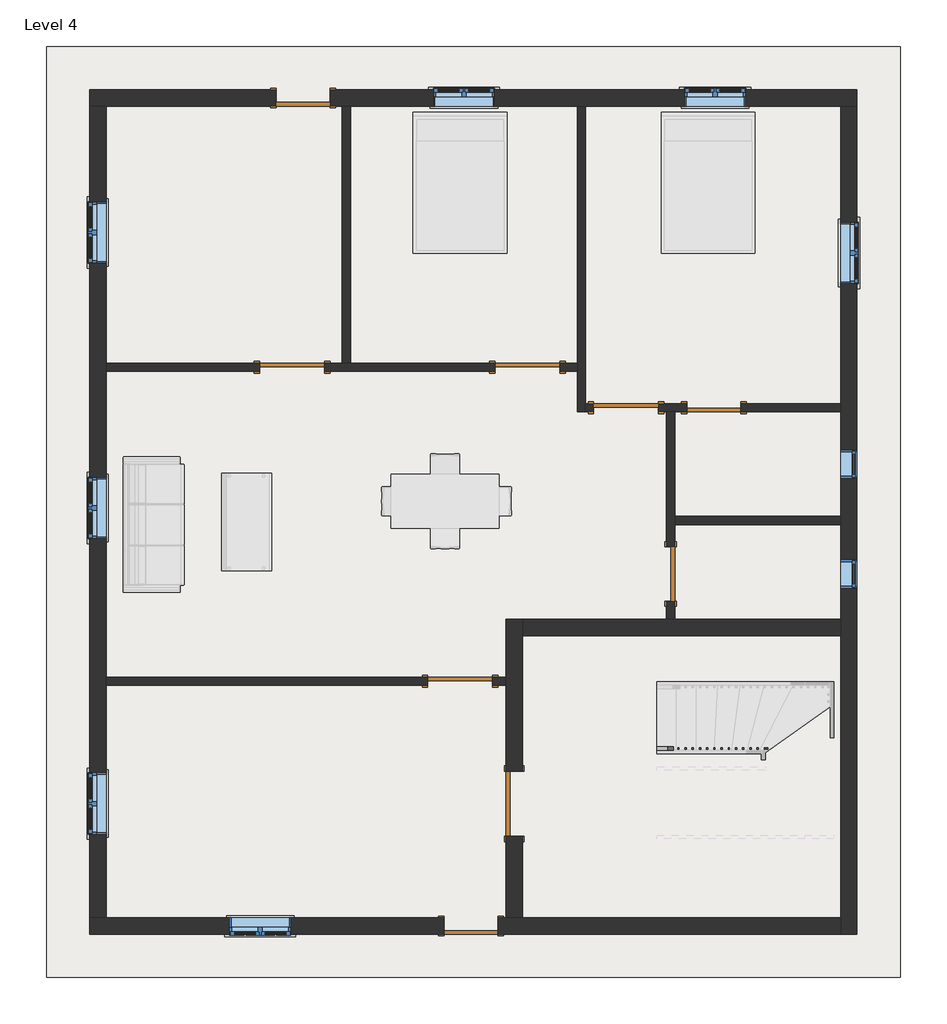
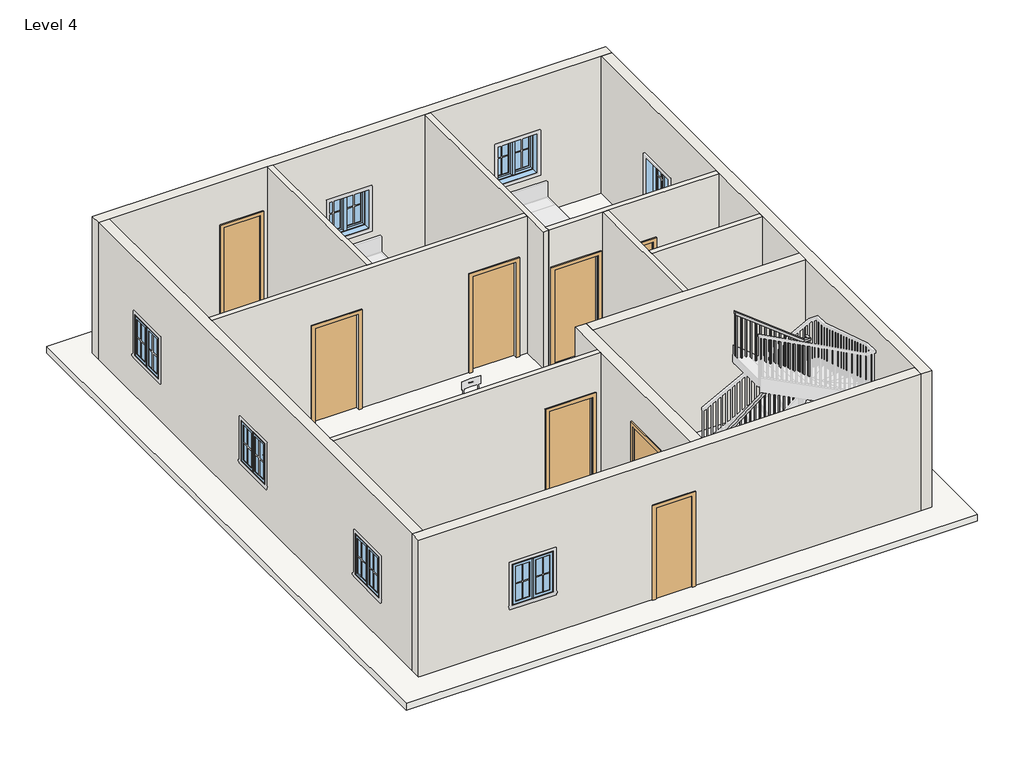
# One storey, part 1 of 2: 13 walls, 9 doors, 9 windows, 1 railing, 1 roof.
"""IFC4 building model written with IfcOpenShell, lengths in millimetres."""

from ifc_helpers import new_model, si_unit, frame, origin, place, context, project, spatial, polyline, outline, extrude, faceted_brep, transform, mapped, element, save
from components import door_85036156, door_d8f5dbb5, door_a1484949, door_e5f9f3c4, door_305aa2a5, door_0ca8825f, window_aa618e30, window_339605e1

model = new_model("IFC4")

# Units and contexts
model_context = context("Model", 3, world=origin())
ifc_project = project(units=[si_unit("LENGTHUNIT", "METRE", prefix="MILLI")], contexts=[model_context])

# Site, building, storey
site = spatial("IfcSite", under=ifc_project)
building = spatial("IfcBuilding", under=site)
storey = spatial("IfcBuildingStorey", under=building, Name="Level 4", Elevation=6400.8)

# Doors
placement = place(None, origin())
door_shape = door_85036156(model_context)
element("IfcDoor", 1, ObjectType="Single-Flush : 30\" x 80\"", at=placement, inside=storey, context=model_context, shape_type="MappedRepresentation", body=[
    mapped(door_shape, transform((-3639.3817864, 7024.9034997, 6400.8), x_axis=(1.0, 0.0, 0.0), y_axis=(0.0, 1.0, 0.0), z_axis=(0.0, 0.0, 1.0))),
])
door_2_shape = door_d8f5dbb5(model_context)
element("IfcDoor", 2, ObjectType="Single-Flush : 30\" x 80\"", at=placement, inside=storey, context=model_context, shape_type="MappedRepresentation", body=[
    mapped(door_2_shape, transform((2149.2782136, 2662.4534997, 6400.8), x_axis=(-1.0, 0.0, 0.0), y_axis=(0.0, -1.0, 0.0), z_axis=(0.0, 0.0, 1.0))),
])
element("IfcDoor", 3, ObjectType="Single-Flush : 30\" x 80\"", at=placement, inside=storey, context=model_context, shape_type="MappedRepresentation", body=[
    mapped(door_2_shape, transform((1539.6782136, 322.4784997, 6400.8), x_axis=(0.0, -1.0, 0.0), y_axis=(1.0, 0.0, 0.0), z_axis=(0.0, 0.0, 1.0))),
])
door_3_shape = door_a1484949(model_context)
element("IfcDoor", 4, ObjectType="Single-Flush : 30\" x 80\"", at=placement, inside=storey, context=model_context, shape_type="MappedRepresentation", body=[
    mapped(door_3_shape, transform((-1273.3717864, -4633.6965003, 6400.8), x_axis=(-1.0, 0.0, 0.0), y_axis=(0.0, -1.0, 0.0), z_axis=(0.0, 0.0, 1.0))),
])
door_4_shape = door_e5f9f3c4(model_context)
element("IfcDoor", 5, ObjectType="Single-Flush : 36\" x 84\"", at=placement, inside=storey, context=model_context, shape_type="MappedRepresentation", body=[
    mapped(door_4_shape, transform((-477.0817864, 3233.9534997, 6400.8), x_axis=(1.0, 0.0, 0.0), y_axis=(0.0, 1.0, 0.0), z_axis=(0.0, 0.0, 1.0))),
])
element("IfcDoor", 6, ObjectType="Single-Flush : 36\" x 84\"", at=placement, inside=storey, context=model_context, shape_type="MappedRepresentation", body=[
    mapped(door_4_shape, transform((-3791.7817864, 3233.9534997, 6400.8), x_axis=(1.0, 0.0, 0.0), y_axis=(0.0, 1.0, 0.0), z_axis=(0.0, 0.0, 1.0))),
])
element("IfcDoor", 7, ObjectType="Single-Flush : 36\" x 84\"", at=placement, inside=storey, context=model_context, shape_type="MappedRepresentation", body=[
    mapped(door_4_shape, transform((-1425.7717864, -1188.1865003, 6400.8), x_axis=(1.0, 0.0, 0.0), y_axis=(0.0, 1.0, 0.0), z_axis=(0.0, 0.0, 1.0))),
])
door_5_shape = door_305aa2a5(model_context)
element("IfcDoor", 8, ObjectType="Single-Flush : 36\" x 84\"", at=placement, inside=storey, context=model_context, shape_type="MappedRepresentation", body=[
    mapped(door_5_shape, transform((912.2982136, 2662.4534997, 6400.8), x_axis=(-1.0, 0.0, 0.0), y_axis=(0.0, -1.0, 0.0), z_axis=(0.0, 0.0, 1.0))),
])
door_6_shape = door_0ca8825f(model_context)
element("IfcDoor", 9, ObjectType="Single-Flush : 36\" x 84\"", at=placement, inside=storey, context=model_context, shape_type="MappedRepresentation", body=[
    mapped(door_6_shape, transform((-663.7717864, -2910.9415003, 6400.8), x_axis=(0.0, 1.0, 0.0), y_axis=(-1.0, 0.0, 0.0), z_axis=(0.0, 0.0, 1.0))),
])

# Railing
element("IfcRailing", 10, ObjectType="Handrail - Rectangular", at=placement, inside=storey, context=model_context, shape_type="SolidModel", body=[
    faceted_brep([(1342.8282136, -2108.9365003, 7484.5333333), (1342.8282136, -2108.9365003, 7420.2000346), (1342.8282136, -2159.7365003, 7420.2000346), (1342.8282136, -2159.7365003, 7484.5333333), (2794.3599055, -2108.9365003, 8612.4191036), (2845.1599055, -2108.9365003, 8587.5590024), (2845.1599055, -2159.7365003, 8587.5590024), (2794.3599055, -2159.7365003, 8612.4191036), (2794.3599055, -2108.9365003, 8815.4281882), (2845.1599055, -2108.9365003, 8764.6281882), (2845.1599055, -2159.7365003, 8764.6281882), (2794.3599055, -2159.7365003, 8815.4281882), (2921.3599055, -2108.9365003, 8815.4281882), (2921.3599055, -2108.9365003, 8764.6281882), (2870.5599055, -2159.7365003, 8764.6281882), (2870.5599055, -2159.7365003, 8815.4281882), (2921.3599055, -2235.9365003, 8815.4281882), (2921.3599055, -2265.0578342, 8764.6281882), (2870.5599055, -2265.0578342, 8764.6281882), (2870.5599055, -2235.9365003, 8815.4281882), (2921.3599055, -2362.9365003, 9032.3051451), (2921.3599055, -2413.7365003, 9018.5256424), (2870.5599055, -2413.7365003, 9018.5256424), (2870.5599055, -2362.9365003, 9032.3051451), (2921.3599055, -2362.9365003, 9235.3142297), (2921.3599055, -2413.7365003, 9184.5142297), (2870.5599055, -2413.7365003, 9184.5142297), (2870.5599055, -2362.9365003, 9235.3142297), (2921.3599055, -2489.9365003, 9235.3142297), (2921.3599055, -2489.9365003, 9184.5142297), (2870.5599055, -2439.1365003, 9184.5142297), (2870.5599055, -2439.1365003, 9235.3142297), (2794.3599055, -2489.9365003, 9235.3142297), (2776.9432376, -2489.9365003, 9184.5142297), (2776.9432376, -2439.1365003, 9184.5142297), (2794.3599055, -2439.1365003, 9235.3142297), (1342.8282136, -2489.9365003, 10363.2), (1342.8282136, -2439.1365003, 10363.2), (1342.8282136, -2439.1365003, 10298.8667013), (1342.8282136, -2489.9365003, 10298.8667013)], [[[0, 1, 2, 3]], [[1, 0, 4, 5]], [[2, 1, 5, 6]], [[3, 2, 6, 7]], [[0, 3, 7, 4]], [[5, 4, 8, 9]], [[6, 5, 9, 10]], [[7, 6, 10, 11]], [[4, 7, 11, 8]], [[9, 8, 12, 13]], [[10, 9, 13, 14]], [[11, 10, 14, 15]], [[8, 11, 15, 12]], [[13, 12, 16, 17]], [[14, 13, 17, 18]], [[15, 14, 18, 19]], [[12, 15, 19, 16]], [[17, 16, 20, 21]], [[18, 17, 21, 22]], [[19, 18, 22, 23]], [[16, 19, 23, 20]], [[21, 20, 24, 25]], [[22, 21, 25, 26]], [[23, 22, 26, 27]], [[20, 23, 27, 24]], [[25, 24, 28, 29]], [[26, 25, 29, 30]], [[27, 26, 30, 31]], [[24, 27, 31, 28]], [[29, 28, 32, 33]], [[30, 29, 33, 34]], [[31, 30, 34, 35]], [[28, 31, 35, 32]], [[36, 37, 38, 39]], [[33, 32, 36, 39]], [[34, 33, 39, 38]], [[35, 34, 38, 37]], [[32, 35, 37, 36]]]),
    extrude(outline(polyline([(10268.8292361, 1381.4849055), (10283.6316852, 1362.4349055), (9279.4666667, 1362.4349055), (9279.4666667, 1381.4849055), (10268.8292361, 1381.4849055)])), frame((0.0, -2474.0615003, 0.0), z_axis=(0.0, 1.0, 0.0), x_axis=(0.0, 0.0, 1.0)), (0.0, 0.0, 1.0), 19.05),
    extrude(outline(polyline([(10189.8828411, 1483.0849055), (10204.6852902, 1464.0349055), (9279.4666667, 1464.0349055), (9279.4666667, 1483.0849055), (10189.8828411, 1483.0849055)])), frame((0.0, -2474.0615003, 0.0), z_axis=(0.0, 1.0, 0.0), x_axis=(0.0, 0.0, 1.0)), (0.0, 0.0, 1.0), 19.05),
    extrude(outline(polyline([(10110.9364462, 1584.6849055), (10125.7388952, 1565.6349055), (9279.4666667, 1565.6349055), (9279.4666667, 1584.6849055), (10110.9364462, 1584.6849055)])), frame((0.0, -2474.0615003, 0.0), z_axis=(0.0, 1.0, 0.0), x_axis=(0.0, 0.0, 1.0)), (0.0, 0.0, 1.0), 19.05),
    extrude(outline(polyline([(10031.9900512, 1686.2849055), (10046.7925003, 1667.2349055), (9110.1333333, 1667.2349055), (9110.1333333, 1686.2849055), (10031.9900512, 1686.2849055)])), frame((0.0, -2474.0615003, 0.0), z_axis=(0.0, 1.0, 0.0), x_axis=(0.0, 0.0, 1.0)), (0.0, 0.0, 1.0), 19.05),
    extrude(outline(polyline([(9953.0436562, 1787.8849055), (9967.8461053, 1768.8349055), (9110.1333333, 1768.8349055), (9110.1333333, 1787.8849055), (9953.0436562, 1787.8849055)])), frame((0.0, -2474.0615003, 0.0), z_axis=(0.0, 1.0, 0.0), x_axis=(0.0, 0.0, 1.0)), (0.0, 0.0, 1.0), 19.05),
    extrude(outline(polyline([(9874.0972613, 1889.4849055), (9888.8997103, 1870.4349055), (9110.1333333, 1870.4349055), (9110.1333333, 1889.4849055), (9874.0972613, 1889.4849055)])), frame((0.0, -2474.0615003, 0.0), z_axis=(0.0, 1.0, 0.0), x_axis=(0.0, 0.0, 1.0)), (0.0, 0.0, 1.0), 19.05),
    extrude(outline(polyline([(9795.1508663, 1991.0849055), (9809.9533154, 1972.0349055), (8940.8, 1972.0349055), (8940.8, 1991.0849055), (9795.1508663, 1991.0849055)])), frame((0.0, -2474.0615003, 0.0), z_axis=(0.0, 1.0, 0.0), x_axis=(0.0, 0.0, 1.0)), (0.0, 0.0, 1.0), 19.05),
    extrude(outline(polyline([(9716.2044713, 2092.6849055), (9731.0069204, 2073.6349055), (8940.8, 2073.6349055), (8940.8, 2092.6849055), (9716.2044713, 2092.6849055)])), frame((0.0, -2474.0615003, 0.0), z_axis=(0.0, 1.0, 0.0), x_axis=(0.0, 0.0, 1.0)), (0.0, 0.0, 1.0), 19.05),
    extrude(outline(polyline([(9637.2580764, 2194.2849055), (9652.0605254, 2175.2349055), (8771.4666667, 2175.2349055), (8771.4666667, 2194.2849055), (9637.2580764, 2194.2849055)])), frame((0.0, -2474.0615003, 0.0), z_axis=(0.0, 1.0, 0.0), x_axis=(0.0, 0.0, 1.0)), (0.0, 0.0, 1.0), 19.05),
    extrude(outline(polyline([(9558.3116814, 2295.8849055), (9573.1141304, 2276.8349055), (8771.4666667, 2276.8349055), (8771.4666667, 2295.8849055), (9558.3116814, 2295.8849055)])), frame((0.0, -2474.0615003, 0.0), z_axis=(0.0, 1.0, 0.0), x_axis=(0.0, 0.0, 1.0)), (0.0, 0.0, 1.0), 19.05),
    extrude(outline(polyline([(9479.3652864, 2397.4849055), (9494.1677355, 2378.4349055), (8771.4666667, 2378.4349055), (8771.4666667, 2397.4849055), (9479.3652864, 2397.4849055)])), frame((0.0, -2474.0615003, 0.0), z_axis=(0.0, 1.0, 0.0), x_axis=(0.0, 0.0, 1.0)), (0.0, 0.0, 1.0), 19.05),
    extrude(outline(polyline([(9400.4188914, 2499.0849055), (9415.2213405, 2480.0349055), (8602.1333333, 2480.0349055), (8602.1333333, 2499.0849055), (9400.4188914, 2499.0849055)])), frame((0.0, -2474.0615003, 0.0), z_axis=(0.0, 1.0, 0.0), x_axis=(0.0, 0.0, 1.0)), (0.0, 0.0, 1.0), 19.05),
    extrude(outline(polyline([(9321.4724965, 2600.6849055), (9336.2749455, 2581.6349055), (8602.1333333, 2581.6349055), (8602.1333333, 2600.6849055), (9321.4724965, 2600.6849055)])), frame((0.0, -2474.0615003, 0.0), z_axis=(0.0, 1.0, 0.0), x_axis=(0.0, 0.0, 1.0)), (0.0, 0.0, 1.0), 19.05),
    extrude(outline(polyline([(9242.5261015, 2702.2849055), (9257.3285506, 2683.2349055), (8432.8, 2683.2349055), (8432.8, 2702.2849055), (9242.5261015, 2702.2849055)])), frame((0.0, -2474.0615003, 0.0), z_axis=(0.0, 1.0, 0.0), x_axis=(0.0, 0.0, 1.0)), (0.0, 0.0, 1.0), 19.05),
    extrude(outline(polyline([(9163.5797065, 2803.8849055), (9178.3821556, 2784.8349055), (8432.8, 2784.8349055), (8432.8, 2803.8849055), (9163.5797065, 2803.8849055)])), frame((0.0, -2474.0615003, 0.0), z_axis=(0.0, 1.0, 0.0), x_axis=(0.0, 0.0, 1.0)), (0.0, 0.0, 1.0), 19.05),
    extrude(outline(polyline([(2886.4349055, -2429.6115003), (2905.4849055, -2429.6115003), (2905.4849055, -2448.6615003), (2886.4349055, -2448.6615003), (2886.4349055, -2429.6115003)])), frame((0.0, 0.0, 8094.1333333), z_axis=(0.0, 0.0, 1.0), x_axis=(1.0, 0.0, 0.0)), (0.0, 0.0, 1.0), 1090.3808964),
    extrude(outline(polyline([(-2347.0615003, 8904.66524), (-2328.0115003, 8872.1336964), (-2328.0115003, 7924.8), (-2347.0615003, 7924.8), (-2347.0615003, 8904.66524)])), frame((2886.4349055, 0.0, 0.0), z_axis=(1.0, 0.0, 0.0), x_axis=(0.0, 1.0, 0.0)), (0.0, 0.0, 1.0), 19.05),
    extrude(outline(polyline([(-2245.4615003, 8731.1636744), (-2226.4115003, 8698.6321309), (-2226.4115003, 7755.4666667), (-2245.4615003, 7755.4666667), (-2245.4615003, 8731.1636744)])), frame((2886.4349055, 0.0, 0.0), z_axis=(1.0, 0.0, 0.0), x_axis=(0.0, 1.0, 0.0)), (0.0, 0.0, 1.0), 19.05),
    extrude(outline(polyline([(2857.3032136, -2143.8615003), (2857.3032136, -2124.8115003), (2876.3532136, -2124.8115003), (2876.3532136, -2143.8615003), (2857.3032136, -2143.8615003)])), frame((0.0, 0.0, 7586.1333333), z_axis=(0.0, 0.0, 1.0), x_axis=(1.0, 0.0, 0.0)), (0.0, 0.0, 1.0), 1178.4948549),
    extrude(outline(polyline([(8532.8507888, 2774.7532136), (8518.0483397, 2755.7032136), (7416.8, 2755.7032136), (7416.8, 2774.7532136), (8532.8507888, 2774.7532136)])), frame((0.0, -2143.8615003, 0.0), z_axis=(0.0, 1.0, 0.0), x_axis=(0.0, 0.0, 1.0)), (0.0, 0.0, 1.0), 19.05),
    extrude(outline(polyline([(8453.9043938, 2673.1532136), (8439.1019447, 2654.1032136), (7416.8, 2654.1032136), (7416.8, 2673.1532136), (8453.9043938, 2673.1532136)])), frame((0.0, -2143.8615003, 0.0), z_axis=(0.0, 1.0, 0.0), x_axis=(0.0, 0.0, 1.0)), (0.0, 0.0, 1.0), 19.05),
    extrude(outline(polyline([(8374.9579988, 2571.5532136), (8360.1555498, 2552.5032136), (7247.4666667, 2552.5032136), (7247.4666667, 2571.5532136), (8374.9579988, 2571.5532136)])), frame((0.0, -2143.8615003, 0.0), z_axis=(0.0, 1.0, 0.0), x_axis=(0.0, 0.0, 1.0)), (0.0, 0.0, 1.0), 19.05),
    extrude(outline(polyline([(8296.0116039, 2469.9532136), (8281.2091548, 2450.9032136), (7247.4666667, 2450.9032136), (7247.4666667, 2469.9532136), (8296.0116039, 2469.9532136)])), frame((0.0, -2143.8615003, 0.0), z_axis=(0.0, 1.0, 0.0), x_axis=(0.0, 0.0, 1.0)), (0.0, 0.0, 1.0), 19.05),
    extrude(outline(polyline([(8217.0652089, 2368.3532136), (8202.2627598, 2349.3032136), (7078.1333333, 2349.3032136), (7078.1333333, 2368.3532136), (8217.0652089, 2368.3532136)])), frame((0.0, -2143.8615003, 0.0), z_axis=(0.0, 1.0, 0.0), x_axis=(0.0, 0.0, 1.0)), (0.0, 0.0, 1.0), 19.05),
    extrude(outline(polyline([(8138.1188139, 2266.7532136), (8123.3163649, 2247.7032136), (7078.1333333, 2247.7032136), (7078.1333333, 2266.7532136), (8138.1188139, 2266.7532136)])), frame((0.0, -2143.8615003, 0.0), z_axis=(0.0, 1.0, 0.0), x_axis=(0.0, 0.0, 1.0)), (0.0, 0.0, 1.0), 19.05),
    extrude(outline(polyline([(8059.1724189, 2165.1532136), (8044.3699699, 2146.1032136), (6908.8, 2146.1032136), (6908.8, 2165.1532136), (8059.1724189, 2165.1532136)])), frame((0.0, -2143.8615003, 0.0), z_axis=(0.0, 1.0, 0.0), x_axis=(0.0, 0.0, 1.0)), (0.0, 0.0, 1.0), 19.05),
    extrude(outline(polyline([(7980.226024, 2063.5532136), (7965.4235749, 2044.5032136), (6908.8, 2044.5032136), (6908.8, 2063.5532136), (7980.226024, 2063.5532136)])), frame((0.0, -2143.8615003, 0.0), z_axis=(0.0, 1.0, 0.0), x_axis=(0.0, 0.0, 1.0)), (0.0, 0.0, 1.0), 19.05),
    extrude(outline(polyline([(7901.279629, 1961.9532136), (7886.4771799, 1942.9032136), (6908.8, 1942.9032136), (6908.8, 1961.9532136), (7901.279629, 1961.9532136)])), frame((0.0, -2143.8615003, 0.0), z_axis=(0.0, 1.0, 0.0), x_axis=(0.0, 0.0, 1.0)), (0.0, 0.0, 1.0), 19.05),
    extrude(outline(polyline([(7822.333234, 1860.3532136), (7807.530785, 1841.3032136), (6739.4666667, 1841.3032136), (6739.4666667, 1860.3532136), (7822.333234, 1860.3532136)])), frame((0.0, -2143.8615003, 0.0), z_axis=(0.0, 1.0, 0.0), x_axis=(0.0, 0.0, 1.0)), (0.0, 0.0, 1.0), 19.05),
    extrude(outline(polyline([(7743.3868391, 1758.7532136), (7728.58439, 1739.7032136), (6739.4666667, 1739.7032136), (6739.4666667, 1758.7532136), (7743.3868391, 1758.7532136)])), frame((0.0, -2143.8615003, 0.0), z_axis=(0.0, 1.0, 0.0), x_axis=(0.0, 0.0, 1.0)), (0.0, 0.0, 1.0), 19.05),
    extrude(outline(polyline([(7664.4404441, 1657.1532136), (7649.637995, 1638.1032136), (6739.4666667, 1638.1032136), (6739.4666667, 1657.1532136), (7664.4404441, 1657.1532136)])), frame((0.0, -2143.8615003, 0.0), z_axis=(0.0, 1.0, 0.0), x_axis=(0.0, 0.0, 1.0)), (0.0, 0.0, 1.0), 19.05),
    extrude(outline(polyline([(7585.4940491, 1555.5532136), (7570.6916001, 1536.5032136), (6570.1333333, 1536.5032136), (6570.1333333, 1555.5532136), (7585.4940491, 1555.5532136)])), frame((0.0, -2143.8615003, 0.0), z_axis=(0.0, 1.0, 0.0), x_axis=(0.0, 0.0, 1.0)), (0.0, 0.0, 1.0), 19.05),
    extrude(outline(polyline([(7506.5476541, 1453.9532136), (7491.7452051, 1434.9032136), (6570.1333333, 1434.9032136), (6570.1333333, 1453.9532136), (7506.5476541, 1453.9532136)])), frame((0.0, -2143.8615003, 0.0), z_axis=(0.0, 1.0, 0.0), x_axis=(0.0, 0.0, 1.0)), (0.0, 0.0, 1.0), 19.05),
    extrude(outline(polyline([(2886.4349055, -2455.0115003), (2905.4849055, -2455.0115003), (2905.4849055, -2474.0615003), (2886.4349055, -2474.0615003), (2886.4349055, -2455.0115003)])), frame((0.0, 0.0, 8263.4666667), z_axis=(0.0, 0.0, 1.0), x_axis=(1.0, 0.0, 0.0)), (0.0, 0.0, 1.0), 921.0475631),
    extrude(outline(polyline([(2886.4349055, -2143.8615003), (2886.4349055, -2124.8115003), (2905.4849055, -2124.8115003), (2905.4849055, -2143.8615003), (2886.4349055, -2143.8615003)])), frame((0.0, 0.0, 7586.1333333), z_axis=(0.0, 0.0, 1.0), x_axis=(1.0, 0.0, 0.0)), (0.0, 0.0, 1.0), 1178.4948549),
    extrude(outline(polyline([(10284.0642523, 1361.8782136), (10298.8667013, 1342.8282136), (9279.4666667, 1342.8282136), (9279.4666667, 1361.8782136), (10284.0642523, 1361.8782136)])), frame((0.0, -2474.0615003, 0.0), z_axis=(0.0, 1.0, 0.0), x_axis=(0.0, 0.0, 1.0)), (0.0, 0.0, 1.0), 19.05),
    extrude(outline(polyline([(7435.0024837, 1361.8782136), (7420.2000346, 1342.8282136), (6570.1333333, 1342.8282136), (6570.1333333, 1361.8782136), (7435.0024837, 1361.8782136)])), frame((0.0, -2143.8615003, 0.0), z_axis=(0.0, 1.0, 0.0), x_axis=(0.0, 0.0, 1.0)), (0.0, 0.0, 1.0), 19.05),
])

# Roof
element("IfcRoof", 11, ObjectType="Generic - 12\"", at=placement, inside=storey, context=model_context, shape_type="SweptSolid", body=[
    extrude(outline(polyline([(-7252.5317864, 7748.8034997), (4771.8282136, 7748.8034997), (4771.8282136, -5357.5965003), (-7252.5317864, -5357.5965003), (-7252.5317864, 7748.8034997)])), frame((0.0, 0.0, 6248.4), z_axis=(0.0, 0.0, 1.0), x_axis=(1.0, 0.0, 0.0)), (0.0, 0.0, 1.0), 152.4),
])

# Walls
element("IfcWall", 12, ObjectType="WALL4.5\"", at=placement, inside=storey, context=model_context, shape_type="Brep", body=[
    faceted_brep([(-3334.5817864, 3176.8034997, 8534.4), (-3334.5817864, 3176.8034997, 6400.8), (-934.2817864, 3176.8034997, 6400.8), (-934.2817864, 3176.8034997, 8534.4), (-19.8817864, 3176.8034997, 8534.4), (-19.8817864, 3176.8034997, 6400.8), (227.7682136, 3176.8034997, 6400.8), (227.7682136, 3176.8034997, 9448.8), (-6414.3317864, 3176.8034997, 9448.8), (-6414.3317864, 3176.8034997, 6400.8), (-4248.9817864, 3176.8034997, 6400.8), (-4248.9817864, 3176.8034997, 8534.4), (-934.2817864, 3291.1034997, 6400.8), (-2972.6317864, 3291.1034997, 6400.8), (-3086.9317864, 3291.1034997, 6400.8), (-3334.5817864, 3291.1034997, 6400.8), (-3334.5817864, 3291.1034997, 8534.4), (-4248.9817864, 3291.1034997, 8534.4), (-4248.9817864, 3291.1034997, 6400.8), (-6414.3317864, 3291.1034997, 6400.8), (-6414.3317864, 3291.1034997, 9448.8), (-3086.9317864, 3291.1034997, 9448.8), (-2972.6317864, 3291.1034997, 9448.8), (227.7682136, 3291.1034997, 9448.8), (227.7682136, 3291.1034997, 6400.8), (-19.8817864, 3291.1034997, 6400.8), (-19.8817864, 3291.1034997, 8534.4), (-934.2817864, 3291.1034997, 8534.4)], [[[0, 1, 2, 3, 4, 5, 6, 7, 8, 9, 10, 11]], [[12, 13, 14, 15, 16, 17, 18, 19, 20, 21, 22, 23, 24, 25, 26, 27]], [[6, 5, 25, 24]], [[10, 9, 19, 18]], [[2, 1, 15, 14, 13, 12]], [[9, 8, 20, 19]], [[7, 6, 24, 23]], [[26, 25, 5, 4]], [[27, 26, 4, 3]], [[12, 27, 3, 2]], [[16, 15, 1, 0]], [[17, 16, 0, 11]], [[18, 17, 11, 10]], [[8, 7, 23, 22, 21, 20]]]),
])
element("IfcWall", 13, ObjectType="WALL4.5\"", at=placement, inside=storey, context=model_context, shape_type="Brep", body=[
    faceted_brep([(227.7682136, 6910.6034997, 6400.8), (227.7682136, 3291.1034997, 6400.8), (227.7682136, 3176.8034997, 6400.8), (227.7682136, 2605.3034997, 6400.8), (227.7682136, 2605.3034997, 9448.8), (227.7682136, 3176.8034997, 9448.8), (227.7682136, 3291.1034997, 9448.8), (227.7682136, 6910.6034997, 9448.8), (342.0682136, 6910.6034997, 6400.8), (342.0682136, 6910.6034997, 9448.8), (342.0682136, 2719.6034997, 9448.8), (342.0682136, 2605.3034997, 9448.8), (342.0682136, 2605.3034997, 6400.8), (342.0682136, 2719.6034997, 6400.8)], [[[0, 1, 2, 3, 4, 5, 6, 7]], [[8, 9, 10, 11, 12, 13]], [[3, 2, 1, 0, 8, 13, 12]], [[0, 7, 9, 8]], [[4, 3, 12, 11]], [[7, 6, 5, 4, 11, 10, 9]]]),
])
element("IfcWall", 14, ObjectType="WALL4.5\"", at=placement, inside=storey, context=model_context, shape_type="Brep", body=[
    faceted_brep([(1369.4982136, 2605.3034997, 6400.8), (1482.5282136, 2605.3034997, 6400.8), (1596.8282136, 2605.3034997, 6400.8), (1768.2782136, 2605.3034997, 6400.8), (1768.2782136, 2605.3034997, 8432.8), (2530.2782136, 2605.3034997, 8432.8), (2530.2782136, 2605.3034997, 6400.8), (3933.6282136, 2605.3034997, 6400.8), (3933.6282136, 2605.3034997, 9448.8), (1596.8282136, 2605.3034997, 9448.8), (1482.5282136, 2605.3034997, 9448.8), (342.0682136, 2605.3034997, 9448.8), (342.0682136, 2605.3034997, 6400.8), (455.0982136, 2605.3034997, 6400.8), (455.0982136, 2605.3034997, 8534.4), (1369.4982136, 2605.3034997, 8534.4), (1768.2782136, 2719.6034997, 8432.8), (1768.2782136, 2719.6034997, 6400.8), (1369.4982136, 2719.6034997, 6400.8), (1369.4982136, 2719.6034997, 8534.4), (455.0982136, 2719.6034997, 8534.4), (455.0982136, 2719.6034997, 6400.8), (342.0682136, 2719.6034997, 6400.8), (342.0682136, 2719.6034997, 9448.8), (3933.6282136, 2719.6034997, 9448.8), (3933.6282136, 2719.6034997, 6400.8), (2530.2782136, 2719.6034997, 6400.8), (2530.2782136, 2719.6034997, 8432.8)], [[[0, 1, 2, 3, 4, 5, 6, 7, 8, 9, 10, 11, 12, 13, 14, 15]], [[16, 17, 18, 19, 20, 21, 22, 23, 24, 25, 26, 27]], [[22, 21, 13, 12]], [[26, 25, 7, 6]], [[18, 17, 3, 2, 1, 0]], [[12, 11, 23, 22]], [[8, 7, 25, 24]], [[14, 13, 21, 20]], [[15, 14, 20, 19]], [[0, 15, 19, 18]], [[4, 3, 17, 16]], [[5, 4, 16, 27]], [[6, 5, 27, 26]], [[11, 10, 9, 8, 24, 23]]]),
])
element("IfcWall", 15, ObjectType="WALL4.5\"", at=placement, inside=storey, context=model_context, shape_type="SweptSolid", body=[
    extrude(outline(polyline([(-3086.9317864, 3291.1034997), (-3086.9317864, 6910.6034997), (-2972.6317864, 6910.6034997), (-2972.6317864, 3291.1034997), (-3086.9317864, 3291.1034997)])), frame((0.0, 0.0, 6400.8), z_axis=(0.0, 0.0, 1.0), x_axis=(1.0, 0.0, 0.0)), (0.0, 0.0, 1.0), 3048.0),
])
element("IfcWall", 16, ObjectType="WALL4.5\"", at=placement, inside=storey, context=model_context, shape_type="Brep", body=[
    faceted_brep([(1482.5282136, -58.5215003, 8432.8), (1482.5282136, -58.5215003, 6400.8), (1482.5282136, -315.6965003, 6400.8), (1482.5282136, -315.6965003, 9448.8), (1482.5282136, 2605.3034997, 9448.8), (1482.5282136, 2605.3034997, 6400.8), (1482.5282136, 703.4784997, 6400.8), (1482.5282136, 703.4784997, 8432.8), (1596.8282136, -315.6965003, 6400.8), (1596.8282136, -58.5215003, 6400.8), (1596.8282136, -58.5215003, 8432.8), (1596.8282136, 703.4784997, 8432.8), (1596.8282136, 703.4784997, 6400.8), (1596.8282136, 1017.8034997, 6400.8), (1596.8282136, 1132.1034997, 6400.8), (1596.8282136, 2605.3034997, 6400.8), (1596.8282136, 2605.3034997, 9448.8), (1596.8282136, 1132.1034997, 9448.8), (1596.8282136, 1017.8034997, 9448.8), (1596.8282136, -315.6965003, 9448.8)], [[[0, 1, 2, 3, 4, 5, 6, 7]], [[8, 9, 10, 11, 12, 13, 14, 15, 16, 17, 18, 19]], [[6, 5, 15, 14, 13, 12]], [[2, 1, 9, 8]], [[5, 4, 16, 15]], [[3, 2, 8, 19]], [[10, 9, 1, 0]], [[11, 10, 0, 7]], [[12, 11, 7, 6]], [[4, 3, 19, 18, 17, 16]]]),
])
element("IfcWall", 17, ObjectType="WALL4.5\"", at=placement, inside=storey, context=model_context, shape_type="SweptSolid", body=[
    extrude(outline(polyline([(3933.6282136, 1017.8034997), (1596.8282136, 1017.8034997), (1596.8282136, 1132.1034997), (3933.6282136, 1132.1034997), (3933.6282136, 1017.8034997)])), frame((0.0, 0.0, 6400.8), z_axis=(0.0, 0.0, 1.0), x_axis=(1.0, 0.0, 0.0)), (0.0, 0.0, 1.0), 3048.0),
])
element("IfcWall", 18, ObjectType="WALL4.5\"", at=placement, inside=storey, context=model_context, shape_type="SweptSolid", body=[
    extrude(outline(polyline([(8534.4, -968.5717864), (6400.8, -968.5717864), (6400.8, -778.0717864), (9448.8, -778.0717864), (9448.8, -6414.3317864), (6400.8, -6414.3317864), (6400.8, -1882.9717864), (8534.4, -1882.9717864), (8534.4, -968.5717864)])), frame((0.0, -1245.3365003, 0.0), z_axis=(0.0, 1.0, 0.0), x_axis=(0.0, 0.0, 1.0)), (0.0, 0.0, 1.0), 114.3),
])
element("IfcWall", 19, ObjectType="WALL9\"", at=placement, inside=storey, context=model_context, shape_type="Brep", body=[
    faceted_brep([(-3258.3817864, 6910.6034997, 8432.8), (-3258.3817864, 6910.6034997, 6400.8), (-3086.9317864, 6910.6034997, 6400.8), (-2972.6317864, 6910.6034997, 6400.8), (227.7682136, 6910.6034997, 6400.8), (342.0682136, 6910.6034997, 6400.8), (3933.6282136, 6910.6034997, 6400.8), (4162.2282136, 6910.6034997, 6400.8), (4162.2282136, 6910.6034997, 9448.8), (3933.6282136, 6910.6034997, 9448.8), (342.0682136, 6910.6034997, 9448.8), (227.7682136, 6910.6034997, 9448.8), (-2972.6317864, 6910.6034997, 9448.8), (-3086.9317864, 6910.6034997, 9448.8), (-6414.3317864, 6910.6034997, 9448.8), (-6642.9317864, 6910.6034997, 9448.8), (-6642.9317864, 6910.6034997, 6400.8), (-6414.3317864, 6910.6034997, 6400.8), (-4020.3817864, 6910.6034997, 6400.8), (-4020.3817864, 6910.6034997, 8432.8), (-940.6317864, 6910.6034997, 8229.6), (-940.6317864, 6910.6034997, 7315.2), (-1804.2317864, 6910.6034997, 7315.2), (-1804.2317864, 6910.6034997, 8229.6), (2598.2232136, 6910.6034997, 8229.6), (2598.2232136, 6910.6034997, 7315.2), (1734.6232136, 6910.6034997, 7315.2), (1734.6232136, 6910.6034997, 8229.6), (4162.2282136, 7139.2034997, 6400.8), (-3258.3817864, 7139.2034997, 6400.8), (-3258.3817864, 7139.2034997, 8432.8), (-4020.3817864, 7139.2034997, 8432.8), (-4020.3817864, 7139.2034997, 6400.8), (-6642.9317864, 7139.2034997, 6400.8), (-6642.9317864, 7139.2034997, 9448.8), (4162.2282136, 7139.2034997, 9448.8), (-940.6317864, 7139.2034997, 8229.6), (-1804.2317864, 7139.2034997, 8229.6), (-1804.2317864, 7139.2034997, 7315.2), (-940.6317864, 7139.2034997, 7315.2), (2598.2232136, 7139.2034997, 8229.6), (1734.6232136, 7139.2034997, 8229.6), (1734.6232136, 7139.2034997, 7315.2), (2598.2232136, 7139.2034997, 7315.2)], [[[0, 1, 2, 3, 4, 5, 6, 7, 8, 9, 10, 11, 12, 13, 14, 15, 16, 17, 18, 19], [20, 21, 22, 23], [24, 25, 26, 27]], [[28, 29, 30, 31, 32, 33, 34, 35], [36, 37, 38, 39], [40, 41, 42, 43]], [[18, 17, 16, 33, 32]], [[7, 6, 5, 4, 3, 2, 1, 29, 28]], [[8, 7, 28, 35]], [[16, 15, 34, 33]], [[30, 29, 1, 0]], [[31, 30, 0, 19]], [[32, 31, 19, 18]], [[21, 20, 36, 39]], [[22, 21, 39, 38]], [[23, 22, 38, 37]], [[20, 23, 37, 36]], [[25, 24, 40, 43]], [[26, 25, 43, 42]], [[27, 26, 42, 41]], [[24, 27, 41, 40]], [[15, 14, 13, 12, 11, 10, 9, 8, 35, 34]]]),
])
element("IfcWall", 20, ObjectType="WALL9\"", at=placement, inside=storey, context=model_context, shape_type="Brep", body=[
    faceted_brep([(3933.6282136, 6910.6034997, 6400.8), (3933.6282136, 2719.6034997, 6400.8), (3933.6282136, 2605.3034997, 6400.8), (3933.6282136, 1132.1034997, 6400.8), (3933.6282136, 1017.8034997, 6400.8), (3933.6282136, -315.6965003, 6400.8), (3933.6282136, -544.2965003, 6400.8), (3933.6282136, -4519.3965003, 6400.8), (3933.6282136, -4747.9965003, 6400.8), (3933.6282136, -4747.9965003, 9448.8), (3933.6282136, -4519.3965003, 9448.8), (3933.6282136, -544.2965003, 9448.8), (3933.6282136, -315.6965003, 9448.8), (3933.6282136, 1017.8034997, 9448.8), (3933.6282136, 1132.1034997, 9448.8), (3933.6282136, 2605.3034997, 9448.8), (3933.6282136, 2719.6034997, 9448.8), (3933.6282136, 6910.6034997, 9448.8), (3933.6282136, 1665.5034997, 7924.8), (3933.6282136, 1665.5034997, 7315.2), (3933.6282136, 2071.9034997, 7315.2), (3933.6282136, 2071.9034997, 7924.8), (3933.6282136, 119.2784997, 7924.8), (3933.6282136, 119.2784997, 7315.2), (3933.6282136, 525.6784997, 7315.2), (3933.6282136, 525.6784997, 7924.8), (3933.6282136, 4411.8784997, 8229.6), (3933.6282136, 4411.8784997, 7315.2), (3933.6282136, 5275.4784997, 7315.2), (3933.6282136, 5275.4784997, 8229.6), (4162.2282136, 6910.6034997, 6400.8), (4162.2282136, 6910.6034997, 9448.8), (4162.2282136, -4747.9965003, 9448.8), (4162.2282136, -4747.9965003, 6400.8), (4162.2282136, 1665.5034997, 7924.8), (4162.2282136, 2071.9034997, 7924.8), (4162.2282136, 2071.9034997, 7315.2), (4162.2282136, 1665.5034997, 7315.2), (4162.2282136, 119.2784997, 7924.8), (4162.2282136, 525.6784997, 7924.8), (4162.2282136, 525.6784997, 7315.2), (4162.2282136, 119.2784997, 7315.2), (4162.2282136, 4411.8784997, 8229.6), (4162.2282136, 5275.4784997, 8229.6), (4162.2282136, 5275.4784997, 7315.2), (4162.2282136, 4411.8784997, 7315.2)], [[[0, 1, 2, 3, 4, 5, 6, 7, 8, 9, 10, 11, 12, 13, 14, 15, 16, 17], [18, 19, 20, 21], [22, 23, 24, 25], [26, 27, 28, 29]], [[30, 31, 32, 33], [34, 35, 36, 37], [38, 39, 40, 41], [42, 43, 44, 45]], [[8, 7, 6, 5, 4, 3, 2, 1, 0, 30, 33]], [[0, 17, 31, 30]], [[9, 8, 33, 32]], [[19, 18, 34, 37]], [[20, 19, 37, 36]], [[21, 20, 36, 35]], [[18, 21, 35, 34]], [[23, 22, 38, 41]], [[24, 23, 41, 40]], [[25, 24, 40, 39]], [[22, 25, 39, 38]], [[27, 26, 42, 45]], [[28, 27, 45, 44]], [[29, 28, 44, 43]], [[26, 29, 43, 42]], [[17, 16, 15, 14, 13, 12, 11, 10, 9, 32, 31]]]),
])
element("IfcWall", 21, ObjectType="WALL9\"", at=placement, inside=storey, context=model_context, shape_type="Brep", body=[
    faceted_brep([(-1654.3717864, -4519.3965003, 8432.8), (-1654.3717864, -4519.3965003, 6400.8), (-6414.3317864, -4519.3965003, 6400.8), (-6642.9317864, -4519.3965003, 6400.8), (-6642.9317864, -4519.3965003, 9448.8), (-6414.3317864, -4519.3965003, 9448.8), (-778.0717864, -4519.3965003, 9448.8), (-549.4717864, -4519.3965003, 9448.8), (3933.6282136, -4519.3965003, 9448.8), (3933.6282136, -4519.3965003, 6400.8), (-549.4717864, -4519.3965003, 6400.8), (-778.0717864, -4519.3965003, 6400.8), (-892.3717864, -4519.3965003, 6400.8), (-892.3717864, -4519.3965003, 8432.8), (-4674.4317864, -4519.3965003, 8229.6), (-4674.4317864, -4519.3965003, 7315.2), (-3810.8317864, -4519.3965003, 7315.2), (-3810.8317864, -4519.3965003, 8229.6), (-6642.9317864, -4747.9965003, 6400.8), (-1654.3717864, -4747.9965003, 6400.8), (-1654.3717864, -4747.9965003, 8432.8), (-892.3717864, -4747.9965003, 8432.8), (-892.3717864, -4747.9965003, 6400.8), (3933.6282136, -4747.9965003, 6400.8), (3933.6282136, -4747.9965003, 9448.8), (-6642.9317864, -4747.9965003, 9448.8), (-4674.4317864, -4747.9965003, 8229.6), (-3810.8317864, -4747.9965003, 8229.6), (-3810.8317864, -4747.9965003, 7315.2), (-4674.4317864, -4747.9965003, 7315.2)], [[[0, 1, 2, 3, 4, 5, 6, 7, 8, 9, 10, 11, 12, 13], [14, 15, 16, 17]], [[18, 19, 20, 21, 22, 23, 24, 25], [26, 27, 28, 29]], [[3, 2, 1, 19, 18]], [[12, 11, 10, 9, 23, 22]], [[9, 8, 24, 23]], [[4, 3, 18, 25]], [[15, 14, 26, 29]], [[16, 15, 29, 28]], [[17, 16, 28, 27]], [[14, 17, 27, 26]], [[8, 7, 6, 5, 4, 25, 24]], [[20, 19, 1, 0]], [[21, 20, 0, 13]], [[22, 21, 13, 12]]]),
])
element("IfcWall", 22, ObjectType="WALL9\"", at=placement, inside=storey, context=model_context, shape_type="Brep", body=[
    faceted_brep([(-6414.3317864, -4519.3965003, 6400.8), (-6414.3317864, -1245.3365003, 6400.8), (-6414.3317864, -1131.0365003, 6400.8), (-6414.3317864, 3176.8034997, 6400.8), (-6414.3317864, 3291.1034997, 6400.8), (-6414.3317864, 6910.6034997, 6400.8), (-6414.3317864, 6910.6034997, 9448.8), (-6414.3317864, 3291.1034997, 9448.8), (-6414.3317864, 3176.8034997, 9448.8), (-6414.3317864, -1131.0365003, 9448.8), (-6414.3317864, -1245.3365003, 9448.8), (-6414.3317864, -4519.3965003, 9448.8), (-6414.3317864, 5561.2284997, 8229.6), (-6414.3317864, 5561.2284997, 7315.2), (-6414.3317864, 4697.6284997, 7315.2), (-6414.3317864, 4697.6284997, 8229.6), (-6414.3317864, 1684.5534997, 8229.6), (-6414.3317864, 1684.5534997, 7315.2), (-6414.3317864, 820.9534997, 7315.2), (-6414.3317864, 820.9534997, 8229.6), (-6414.3317864, -2479.1415003, 8229.6), (-6414.3317864, -2479.1415003, 7315.2), (-6414.3317864, -3342.7415003, 7315.2), (-6414.3317864, -3342.7415003, 8229.6), (-6642.9317864, -4519.3965003, 6400.8), (-6642.9317864, -4519.3965003, 9448.8), (-6642.9317864, 6910.6034997, 9448.8), (-6642.9317864, 6910.6034997, 6400.8), (-6642.9317864, 5561.2284997, 8229.6), (-6642.9317864, 4697.6284997, 8229.6), (-6642.9317864, 4697.6284997, 7315.2), (-6642.9317864, 5561.2284997, 7315.2), (-6642.9317864, 1684.5534997, 8229.6), (-6642.9317864, 820.9534997, 8229.6), (-6642.9317864, 820.9534997, 7315.2), (-6642.9317864, 1684.5534997, 7315.2), (-6642.9317864, -2479.1415003, 8229.6), (-6642.9317864, -3342.7415003, 8229.6), (-6642.9317864, -3342.7415003, 7315.2), (-6642.9317864, -2479.1415003, 7315.2)], [[[0, 1, 2, 3, 4, 5, 6, 7, 8, 9, 10, 11], [12, 13, 14, 15], [16, 17, 18, 19], [20, 21, 22, 23]], [[24, 25, 26, 27], [28, 29, 30, 31], [32, 33, 34, 35], [36, 37, 38, 39]], [[5, 4, 3, 2, 1, 0, 24, 27]], [[0, 11, 25, 24]], [[6, 5, 27, 26]], [[13, 12, 28, 31]], [[14, 13, 31, 30]], [[15, 14, 30, 29]], [[12, 15, 29, 28]], [[17, 16, 32, 35]], [[18, 17, 35, 34]], [[19, 18, 34, 33]], [[16, 19, 33, 32]], [[21, 20, 36, 39]], [[22, 21, 39, 38]], [[23, 22, 38, 37]], [[20, 23, 37, 36]], [[11, 10, 9, 8, 7, 6, 26, 25]]]),
])
element("IfcWall", 23, ObjectType="WALL9\"", at=placement, inside=storey, context=model_context, shape_type="Brep", body=[
    faceted_brep([(-549.4717864, -2453.7415003, 8534.4), (-549.4717864, -2453.7415003, 6400.8), (-549.4717864, -544.2965003, 6400.8), (-549.4717864, -315.6965003, 6400.8), (-549.4717864, -315.6965003, 9448.8), (-549.4717864, -544.2965003, 9448.8), (-549.4717864, -4519.3965003, 9448.8), (-549.4717864, -4519.3965003, 6400.8), (-549.4717864, -3368.1415003, 6400.8), (-549.4717864, -3368.1415003, 8534.4), (-778.0717864, -315.6965003, 6400.8), (-778.0717864, -1131.0365003, 6400.8), (-778.0717864, -1245.3365003, 6400.8), (-778.0717864, -2453.7415003, 6400.8), (-778.0717864, -2453.7415003, 8534.4), (-778.0717864, -3368.1415003, 8534.4), (-778.0717864, -3368.1415003, 6400.8), (-778.0717864, -4519.3965003, 6400.8), (-778.0717864, -4519.3965003, 9448.8), (-778.0717864, -1245.3365003, 9448.8), (-778.0717864, -1131.0365003, 9448.8), (-778.0717864, -315.6965003, 9448.8)], [[[0, 1, 2, 3, 4, 5, 6, 7, 8, 9]], [[10, 11, 12, 13, 14, 15, 16, 17, 18, 19, 20, 21]], [[8, 7, 17, 16]], [[3, 2, 1, 13, 12, 11, 10]], [[7, 6, 18, 17]], [[4, 3, 10, 21]], [[14, 13, 1, 0]], [[15, 14, 0, 9]], [[16, 15, 9, 8]], [[6, 5, 4, 21, 20, 19, 18]]]),
])
element("IfcWall", 24, ObjectType="WALL9\"", at=placement, inside=storey, context=model_context, shape_type="Brep", body=[
    faceted_brep([(-549.4717864, -544.2965003, 6400.8), (3933.6282136, -544.2965003, 6400.8), (3933.6282136, -544.2965003, 9448.8), (-549.4717864, -544.2965003, 9448.8), (-549.4717864, -315.6965003, 6400.8), (-549.4717864, -315.6965003, 9448.8), (1482.5282136, -315.6965003, 9448.8), (1596.8282136, -315.6965003, 9448.8), (3933.6282136, -315.6965003, 9448.8), (3933.6282136, -315.6965003, 6400.8), (1596.8282136, -315.6965003, 6400.8), (1482.5282136, -315.6965003, 6400.8)], [[[0, 1, 2, 3]], [[4, 5, 6, 7, 8, 9, 10, 11]], [[1, 0, 4, 11, 10, 9]], [[0, 3, 5, 4]], [[2, 1, 9, 8]], [[3, 2, 8, 7, 6, 5]]]),
])

# Windows
window_shape = window_aa618e30(model_context)
element("IfcWindow", 25, ObjectType="Fixed : 16\" x 24\"", at=placement, inside=storey, context=model_context, shape_type="MappedRepresentation", body=[
    mapped(window_shape, transform((4047.9282136, 1830.6034997, 6400.8), x_axis=(0.0, -1.0, 0.0), y_axis=(1.0, 0.0, 0.0), z_axis=(0.0, 0.0, 1.0))),
])
element("IfcWindow", 26, ObjectType="Fixed : 16\" x 24\"", at=placement, inside=storey, context=model_context, shape_type="MappedRepresentation", body=[
    mapped(window_shape, transform((4047.9282136, 284.3784997, 6400.8), x_axis=(0.0, -1.0, 0.0), y_axis=(1.0, 0.0, 0.0), z_axis=(0.0, 0.0, 1.0))),
])
window_2_shape = window_339605e1(model_context)
element("IfcWindow", 27, ObjectType="Window-Casement-Double : 34\" x 36\"", at=placement, inside=storey, context=model_context, shape_type="MappedRepresentation", body=[
    mapped(window_2_shape, transform((-1372.4317864, 7024.9034997, 6400.8), x_axis=(1.0, 0.0, 0.0), y_axis=(0.0, 1.0, 0.0), z_axis=(0.0, 0.0, 1.0))),
])
element("IfcWindow", 28, ObjectType="Window-Casement-Double : 34\" x 36\"", at=placement, inside=storey, context=model_context, shape_type="MappedRepresentation", body=[
    mapped(window_2_shape, transform((2166.4232136, 7024.9034997, 6400.8), x_axis=(1.0, 0.0, 0.0), y_axis=(0.0, 1.0, 0.0), z_axis=(0.0, 0.0, 1.0))),
])
element("IfcWindow", 29, ObjectType="Window-Casement-Double : 34\" x 36\"", at=placement, inside=storey, context=model_context, shape_type="MappedRepresentation", body=[
    mapped(window_2_shape, transform((-6528.6317864, 5129.4284997, 6400.8), x_axis=(0.0, 1.0, 0.0), y_axis=(-1.0, 0.0, 0.0), z_axis=(0.0, 0.0, 1.0))),
])
element("IfcWindow", 30, ObjectType="Window-Casement-Double : 34\" x 36\"", at=placement, inside=storey, context=model_context, shape_type="MappedRepresentation", body=[
    mapped(window_2_shape, transform((-6528.6317864, 1252.7534997, 6400.8), x_axis=(0.0, 1.0, 0.0), y_axis=(-1.0, 0.0, 0.0), z_axis=(0.0, 0.0, 1.0))),
])
element("IfcWindow", 31, ObjectType="Window-Casement-Double : 34\" x 36\"", at=placement, inside=storey, context=model_context, shape_type="MappedRepresentation", body=[
    mapped(window_2_shape, transform((4047.9282136, 4843.6784997, 6400.8), x_axis=(0.0, -1.0, 0.0), y_axis=(1.0, 0.0, 0.0), z_axis=(0.0, 0.0, 1.0))),
])
element("IfcWindow", 32, ObjectType="Window-Casement-Double : 34\" x 36\"", at=placement, inside=storey, context=model_context, shape_type="MappedRepresentation", body=[
    mapped(window_2_shape, transform((-6528.6317864, -2910.9415003, 6400.8), x_axis=(0.0, 1.0, 0.0), y_axis=(-1.0, 0.0, 0.0), z_axis=(0.0, 0.0, 1.0))),
])
element("IfcWindow", 33, ObjectType="Window-Casement-Double : 34\" x 36\"", at=placement, inside=storey, context=model_context, shape_type="MappedRepresentation", body=[
    mapped(window_2_shape, transform((-4242.6317864, -4633.6965003, 6400.8), x_axis=(-1.0, 0.0, 0.0), y_axis=(0.0, -1.0, 0.0), z_axis=(0.0, 0.0, 1.0))),
])

save(model, "model.ifc")

# Revit data of these elements
# Type "Single-Flush : 30\" x 80\""
#   Type Mark = "5"
#   Construction Type Id = "MDOOR"
#   Assembly Code = "C1020"
#   Analytic Construction = "Metal"
#   Thickness = 0' - 2"
#   Heat Transfer Coefficient (U) = 0.651978 BTU/(h·ft²·°F)
#   Height = 6' - 8"
#   Trim Projection Ext = 0' - 1"
#   Trim Projection Int = 0' - 1"
#   Trim Width = 0' - 3"
#   Width = 2' - 6"
#   Define Thermal Properties by = 1
#   Define Thermal Properties by = 1
#   Door Material = Door - Panel
#   Frame Material = Door - Frame
#   Visual Light Transmittance = 0
#   Solar Heat Gain Coefficient = 0
#   Function = (empty or 0)
#   Wall Closure = (empty or 0)
# Type "Single-Flush : 36\" x 84\""
#   Type Mark = "1"
#   Construction Type Id = "MDOOR"
#   Assembly Code = "C1020"
#   Analytic Construction = "Metal"
#   Thickness = 0' - 2"
#   Heat Transfer Coefficient (U) = 0.651978 BTU/(h·ft²·°F)
#   Height = 7' - 0"
#   Trim Projection Ext = 0' - 1"
#   Trim Projection Int = 0' - 1"
#   Trim Width = 0' - 3"
#   Width = 3' - 0"
#   Define Thermal Properties by = 1
#   Define Thermal Properties by = 1
#   Door Material = Door - Panel
#   Frame Material = Door - Frame
#   Visual Light Transmittance = 0
#   Solar Heat Gain Coefficient = 0
#   Function = (empty or 0)
#   Wall Closure = (empty or 0)
# Type "Handrail - Rectangular"
#   Assembly Code = "C2010400"
#   built-in parameter 1008612 = 0.0416667 (stored number, unit not read)
#   built-in parameter 1008611 = 0.0416667 (stored number, unit not read)
#   built-in parameter 1008609 = 0.333333 (stored number, unit not read)
#   built-in parameter 1008604 = 0.166667 (stored number, unit not read)
#   built-in parameter 1008603 = 0.166667 (stored number, unit not read)
#   Railing Height = 3' - 0"
#   built-in parameter 1008630 = 2
#   built-in parameter 1008610 = 2
#   built-in parameter 1008618 = Baluster - Square : 3/4"
# Type "Generic - 12\""
#   Assembly Code = "B1020"
#   Layers, outside or top first: 0' - 6" no material (function 1)
# Type "WALL4.5\""
#   Assembly Code = "B2010"
#   Layers, outside or top first: 0' - 4 1/2" no material (function 1)
# Type "WALL9\""
#   Assembly Code = "B2010"
#   Layers, outside or top first: 0' - 9" no material (function 1)
# Type "Fixed : 16\" x 24\""
#   Type Mark = "4"
#   Construction Type Id = "GSP4R"
#   Assembly Code = "B2020100"
#   Analytic Construction = "1/8 in Pilkington single glazing"
#   Visual Light Transmittance = 0.9
#   Solar Heat Gain Coefficient = 0.78
#   Heat Transfer Coefficient (U) = 0.6496 BTU/(h·ft²·°F)
#   Height = 2' - 0"
#   Default Sill Height = 3' - 0"
#   Width = 1' - 4"
#   Window Inset = 0' - 0 3/4"
#   Define Thermal Properties by = 1
#   Define Thermal Properties by = 1
#   Glass Pane Material = Glass
#   Sash Material = Sash
#   Wall Closure = (empty or 0)
# Type "Window-Casement-Double : 34\" x 36\""
#   Type Mark = "14"
#   Fire Rating = "0.5h"
#   Assembly Code = "B2020100"
#   Analytic Construction = "Double glazing - domestic"
#   Frame Extension [instance default] = 0' - 0 1/4"
#   Window Inset [instance default] = 0' - 0"
#   Wall Thickness [instance default] = 0' - 6"
#   Interior Wall Closure [instance default] = 0' - 2 1/4"
#   Half Width = 1' - 5"
#   Visual Light Transmittance = 0.81
#   Thermal Resistance (R) = 1.8146 (h·ft²·°F)/BTU
#   Solar Heat Gain Coefficient = 0.76
#   Rough Width = 2' - 10 1/2"
#   Rough Height = 3' - 0 1/2"
#   Height = 3' - 0"
#   Heat Transfer Coefficient (U) = 0.5511 BTU/(h·ft²·°F)
#   Exterior Wall Closure [instance default] = 0' - 1 1/4"
#   Extension Jamb [instance default] = 0' - 2 1/4"
#   Default Sill Height = 3' - 0"
#   Width = 2' - 10"
#   Define Thermal Properties by = 0
#   Muntin Visibility = yes
#   Interior Trim Visibility [instance default] = yes
#   Exterior Trim Visibility [instance default] = yes
#   Extension Jamb Visibility [instance default] = yes
#   Interior Trim Material = Wood - Stained
#   Muntin Pattern = Muntin Pattern_2x2 : Muntin Pattern_2x2
#   Interior Trim = Trim-Window-Interior-Flat : Picture Frame
#   Interior Frame Material = Wood - Stained
#   Glass Panel Material = Glass
#   Exterior Trim Material = Clad - White
#   Exterior Trim = Trim-Window-Exterior-Flat : with Sill
#   Exterior Frame Material = Clad - White
#   Wall Closure = (empty or 0)
# Elements 1, 2, 3, 4 (IfcDoor, "Single-Flush : 30\" x 80\"")
#   Phase Created = New Construction
#   Materials on its faces: "Door - Frame", "Door - Panel"
# Elements 5, 6, 7, 8, 9 (IfcDoor, "Single-Flush : 36\" x 84\"")
#   Phase Created = New Construction
#   Materials on its faces: "Door - Frame", "Door - Panel"
# Element 10 (IfcRailing, "Handrail - Rectangular")
#   Phase Created = New Construction
# Element 11 (IfcRoof, "Generic - 12\"")
#   built-in parameter 1001705 = 21 (stored number, unit not read)
#   built-in parameter 1001701 = -0.5 (stored number, unit not read)
#   built-in parameter 1001710 = 33615
#   Phase Created = New Construction
#   Materials on its faces: "Default Roof", "Wood Planks"
# Elements 12, 13, 14, 15, 16, 17, 18 (IfcWall, "WALL4.5\"")
#   Top Offset = 0' - 0"
#   Base Offset = 0' - 0"
#   Unconnected Height = 10' - 0"
#   wall height = 10' - 0"
#   Phase Created = New Construction
#   Base Constraint = Level 4
#   Materials on its faces: "Default Wall"
# Elements 19, 20, 21, 22 (IfcWall, "WALL9\"")
#   Top Offset = 0' - 0"
#   Base Offset = 0' - 0"
#   Unconnected Height = 10' - 0"
#   wall height = 10' - 0"
#   Phase Created = New Construction
#   Base Constraint = Level 4
#   Materials on its faces: "Default Wall", "Wood Planks"
# Elements 23, 24 (IfcWall, "WALL9\"")
#   Top Offset = 0' - 0"
#   Base Offset = 0' - 0"
#   Unconnected Height = 10' - 0"
#   wall height = 10' - 0"
#   Phase Created = New Construction
#   Base Constraint = Level 4
#   Materials on its faces: "Default Wall"
# Element 25 (IfcWindow, "Fixed : 16\" x 24\"")
#   Mark = "19"
#   Phase Created = New Construction
#   Materials on its faces: "Sash", "Glass"
# Element 26 (IfcWindow, "Fixed : 16\" x 24\"")
#   Mark = "20"
#   Phase Created = New Construction
#   Materials on its faces: "Sash", "Glass"
# Element 27 (IfcWindow, "Window-Casement-Double : 34\" x 36\"")
#   Mark = "21"
#   Window Inset = 0' - 0"
#   Interior Wall Closure = 0' - 2 1/4"
#   Frame Extension = 0' - 0 1/4"
#   Exterior Wall Closure = 0' - 1 1/4"
#   Interior Trim Visibility = yes
#   Exterior Trim Visibility = yes
#   Phase Created = New Construction
#   Materials on its faces: "Wood - Stained", "Glass", "Clad - White"
# Element 28 (IfcWindow, "Window-Casement-Double : 34\" x 36\"")
#   Mark = "22"
#   Window Inset = 0' - 0"
#   Interior Wall Closure = 0' - 2 1/4"
#   Frame Extension = 0' - 0 1/4"
#   Exterior Wall Closure = 0' - 1 1/4"
#   Interior Trim Visibility = yes
#   Exterior Trim Visibility = yes
#   Phase Created = New Construction
#   Materials on its faces: "Wood - Stained", "Glass", "Clad - White"
# Element 29 (IfcWindow, "Window-Casement-Double : 34\" x 36\"")
#   Mark = "23"
#   Window Inset = 0' - 0"
#   Interior Wall Closure = 0' - 2 1/4"
#   Frame Extension = 0' - 0 1/4"
#   Exterior Wall Closure = 0' - 1 1/4"
#   Interior Trim Visibility = yes
#   Exterior Trim Visibility = yes
#   Phase Created = New Construction
#   Materials on its faces: "Wood - Stained", "Glass", "Clad - White"
# Element 30 (IfcWindow, "Window-Casement-Double : 34\" x 36\"")
#   Mark = "24"
#   Window Inset = 0' - 0"
#   Interior Wall Closure = 0' - 2 1/4"
#   Frame Extension = 0' - 0 1/4"
#   Exterior Wall Closure = 0' - 1 1/4"
#   Interior Trim Visibility = yes
#   Exterior Trim Visibility = yes
#   Phase Created = New Construction
#   Materials on its faces: "Wood - Stained", "Glass", "Clad - White"
# Element 31 (IfcWindow, "Window-Casement-Double : 34\" x 36\"")
#   Mark = "25"
#   Window Inset = 0' - 0"
#   Interior Wall Closure = 0' - 2 1/4"
#   Frame Extension = 0' - 0 1/4"
#   Exterior Wall Closure = 0' - 1 1/4"
#   Interior Trim Visibility = yes
#   Exterior Trim Visibility = yes
#   Phase Created = New Construction
#   Materials on its faces: "Wood - Stained", "Glass", "Clad - White"
# Element 32 (IfcWindow, "Window-Casement-Double : 34\" x 36\"")
#   Mark = "26"
#   Window Inset = 0' - 0"
#   Interior Wall Closure = 0' - 2 1/4"
#   Frame Extension = 0' - 0 1/4"
#   Exterior Wall Closure = 0' - 1 1/4"
#   Interior Trim Visibility = yes
#   Exterior Trim Visibility = yes
#   Phase Created = New Construction
#   Materials on its faces: "Wood - Stained", "Glass", "Clad - White"
# Element 33 (IfcWindow, "Window-Casement-Double : 34\" x 36\"")
#   Mark = "27"
#   Window Inset = 0' - 0"
#   Interior Wall Closure = 0' - 2 1/4"
#   Frame Extension = 0' - 0 1/4"
#   Exterior Wall Closure = 0' - 1 1/4"
#   Interior Trim Visibility = yes
#   Exterior Trim Visibility = yes
#   Phase Created = New Construction
#   Materials on its faces: "Wood - Stained", "Glass", "Clad - White"
# Materials
#   "Door - Panel": class "Wood", colour RGB 210 159 95, transparency 0, Cost = 0
#   "Door - Frame": colour RGB 118 70 51, transparency 0, Cost = 0
#   "Glass": class "Glass", colour RGB 0 128 192, transparency 0.75, Description = "Soda Lime Glass", Cost = 0
#   "Sash": class "Wood", colour RGB 224 178 126, transparency 0, Cost = 0
#   "Wood - Stained": class "Wood", colour RGB 224 178 126, transparency 0, Cost = 0
#   "Clad - White": class "Wood", colour RGB 242 242 238, transparency 0, Cost = 0
#   "Default Roof": colour RGB 88 101 114, transparency 0, Cost = 0
#   "Wood Planks": class "Wood", colour RGB 193 160 115, transparency 0, Description = "Physical material.", Cost = 0
#   "Default Wall": colour RGB 128 128 128, transparency 0, Cost = 0
